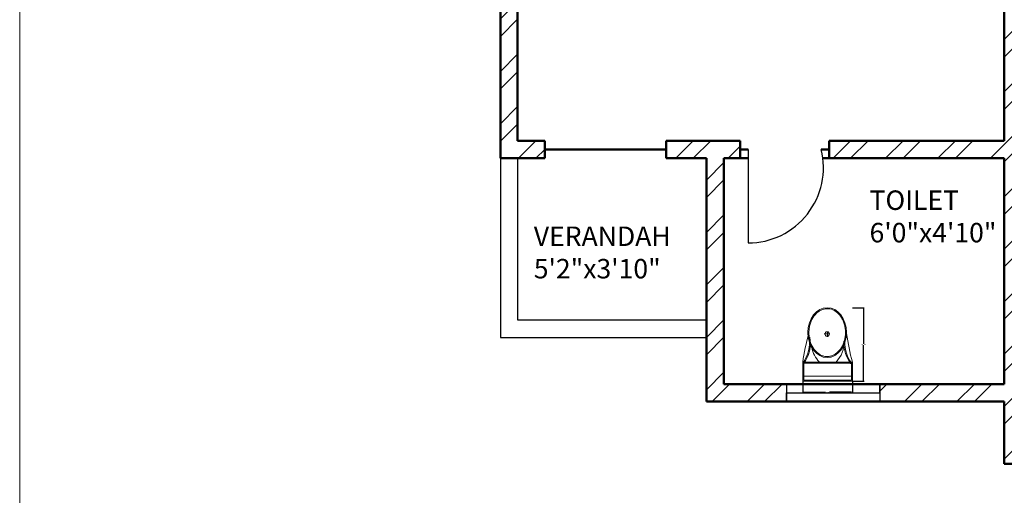
# Model space of a CAD drawing. Units: inches. Extents: x 1901 to 2863, y 888 to 2433.
# Tile 2 of 91: x 1901 to 2154, y 1216 to 1338. Entities that reach past the tile are written whole.
import ezdxf

# ---------------------------------------------------------------- set-up
doc = ezdxf.new("R2010")
doc.units = ezdxf.units.IN
for name, color, linetype, lineweight in [('A-ANNO-DIMS', 2, 'Continuous', 18), ('A-AREA-IDEN', 7, 'Continuous', 18), ('A-DOOR', 4, 'Continuous', 25), ('A-FLOR-FIXT', 9, 'Continuous', 18), ('A-FLOR-HRAL', 41, 'Continuous', 25), ('A-GLAZ', 3, 'Continuous', 25), ('A-WALL', 7, 'Continuous', 50), ('A-WALL-PATT', 8, 'Continuous', 13)]:
    doc.layers.add(name, color=color, linetype=linetype, lineweight=lineweight)
doc.styles.get("Standard").update_dxf_attribs({"font": 'arial.ttf'})
doc.dimstyles.get("Standard").update_dxf_attribs({"dimtxt": 0.18, "dimasz": 0.18, "dimexe": 0.18, "dimexo": 0.0625, "dimgap": 0.09, "dimtad": 0, "dimtih": 1, "dimtoh": 1, "dimdec": 4, "dimzin": 0, "dimdsep": 46, "dimtxsty": 'Standard', "dimcen": 0.09, "dimadec": 0, "dimazin": 0, "dimtfac": 1, "dimtdec": 4, "dimtofl": 0, "dimtmove": 0, "dimatfit": 3, "dimfxl": 1, "dimtolj": 1, "dimtzin": 0, "dimarcsym": 0})

# ---------------------------------------------------------------- blocks, each defined once
blk = doc.blocks.new('A$C31115884')
for p, q in [((258, 466), (258, 523)), ((283, 498), (223, 498)), ((0, 200), (0, 0)), ((520, 200), (0, 200)), ((10, 190), (10, 10)), ((510, 190), (10, 190)), ((510, 10), (510, 190)), ((520, 0), (520, 200)), ((510, 54), (0, 54)), ((10, 10), (510, 10)), ((0, 0), (520, 0))]:
    blk.add_line(p, q)
blk.add_circle((256, 496), 23.6)
for centre, radius, start, end in [((2778, -205), 2807, 165.4549, 171.7133), ((-295, 403), 365, 324.2091, 9.3499), ((-295, 403), 375, 324.2091, 9.3499), ((139, 406), 293, 315.8436, 2.6563), ((806, 403), 365, 170.6501, 215.7909), ((3237, 905), 2807, 188.2867, 194.5451), ((384, 406), 293, 190.2774, 224.1564), ((806, 403), 375, 179.2036, 215.7909)]:
    blk.add_arc(centre, radius, start, end)
blk.add_ellipse((256, 510), major_axis=(0, -261), ratio=0.772727)
blk.add_open_spline([(256, 259), (263, 259), (270, 260), (288, 262), (299, 265), (320, 273), (330, 278), (350, 291), (360, 299), (378, 316), (386, 326), (402, 347), (409, 358), (421, 383), (427, 395), (436, 422), (440, 436), (445, 465), (447, 480), (448, 509), (448, 524), (445, 553), (443, 568), (436, 596), (432, 610), (422, 636), (416, 649), (402, 672), (395, 683), (379, 703), (370, 712), (351, 728), (341, 735), (321, 746), (310, 751), (289, 757), (278, 759), (256, 761), (245, 761), (223, 757), (212, 754), (191, 746), (181, 741), (161, 728), (151, 720), (133, 703), (125, 693), (110, 672), (103, 660), (90, 636), (85, 623), (76, 596), (72, 582), (67, 553), (66, 538), (64, 509), (65, 494), (68, 465), (70, 450), (77, 422), (81, 408), (91, 382), (97, 370), (111, 346), (118, 335), (135, 316), (144, 307), (162, 291), (172, 284), (193, 273), (203, 269), (225, 262), (236, 260), (250, 259), (253, 259), (256, 259)], degree=3, knots=[0, 0, 0, 0, 0.110105, 0.110105, 0.285049, 0.285049, 0.459994, 0.459994, 0.634938, 0.634938, 0.809882, 0.809882, 0.984827, 0.984827, 1.159771, 1.159771, 1.334715, 1.334715, 1.50966, 1.50966, 1.684604, 1.684604, 1.859549, 1.859549, 2.034493, 2.034493, 2.209437, 2.209437, 2.384382, 2.384382, 2.559326, 2.559326, 2.73427, 2.73427, 2.909215, 2.909215, 3.084159, 3.084159, 3.259103, 3.259103, 3.434048, 3.434048, 3.608992, 3.608992, 3.783936, 3.783936, 3.958881, 3.958881, 4.133825, 4.133825, 4.30877, 4.30877, 4.483714, 4.483714, 4.658658, 4.658658, 4.833603, 4.833603, 5.008547, 5.008547, 5.183491, 5.183491, 5.358436, 5.358436, 5.53338, 5.53338, 5.708324, 5.708324, 5.883269, 5.883269, 6.058213, 6.058213, 6.233158, 6.233158, 6.283185, 6.283185, 6.283185, 6.283185])
blk = doc.blocks.new('WIN-24')
for p, q in [((0, 4.5), (0, 0)), ((24, 2.25), (24, 4.5)), ((24, 4.5), (24, 0)), ((0, 0), (0, 2.25)), ((0, 2.25), (24, 2.25))]:
    blk.add_line(p, q)
blk = doc.blocks.new('*D15')
at = {"layer": 'A-ANNO-DIMS', "color": 0, "lineweight": -2, "transparency": 16777216}
for p, q in [((2115.37, 1263.74), (2118.32, 1263.74)), ((2118.14, 1263.56), (2118.14, 1254.48)), ((2118.14, 1245.03), (2118.14, 1254.11)), ((2115.37, 1244.85), (2118.32, 1244.85))]:
    blk.add_line(p, q, dxfattribs=at)
at = {"layer": 'A-ANNO-DIMS', "color": 0, "transparency": 16777216}
for points in [[(2118.11, 1263.56), (2118.17, 1263.56), (2118.14, 1263.74)], [(2118.11, 1245.03), (2118.17, 1245.03), (2118.14, 1244.85)]]:
    blk.add_solid(points, dxfattribs=at)
at = {"layer": 'Defpoints', "color": 0, "transparency": 16777216}
for p in [(2115.3, 1263.74), (2118.14, 1263.74), (2115.3, 1244.85)]:
    blk.add_point(p, dxfattribs=at)
at = {"layer": 'A-ANNO-DIMS', "color": 0, "transparency": 16777216, "insert": (2118.14, 1254.3), "char_height": 0.18, "attachment_point": 5}
blk.add_mtext('\\A1;WC 19 TYP.', dxfattribs=at)
blk = doc.blocks.new('*D16')
at = {"layer": 'A-ANNO-DIMS', "color": 0, "lineweight": -2, "transparency": 16777216}
for p, q in [((2102.56, 1244.79), (2102.56, 1241.84)), ((2115.3, 1244.79), (2115.3, 1241.84)), ((2102.74, 1242.02), (2108.41, 1242.02)), ((2115.12, 1242.02), (2109.45, 1242.02))]:
    blk.add_line(p, q, dxfattribs=at)
at = {"layer": 'A-ANNO-DIMS', "color": 0, "transparency": 16777216}
for points in [[(2102.74, 1242.05), (2102.74, 1241.99), (2102.56, 1242.02)], [(2115.12, 1242.05), (2115.12, 1241.99), (2115.3, 1242.02)]]:
    blk.add_solid(points, dxfattribs=at)
at = {"layer": 'Defpoints', "color": 0, "transparency": 16777216}
for p in [(2102.56, 1244.85), (2115.3, 1244.85), (2115.3, 1242.02)]:
    blk.add_point(p, dxfattribs=at)
at = {"layer": 'A-ANNO-DIMS', "color": 0, "transparency": 16777216, "insert": (2108.93, 1242.02), "char_height": 0.18, "attachment_point": 5}
blk.add_mtext('\\A1;13 TYP.', dxfattribs=at)

msp = doc.modelspace()

# ---------------------------------------------------------------- hatches: boundary and pattern name
at = {"layer": 'A-WALL-PATT'}
h = msp.add_hatch(dxfattribs=at)
h.set_pattern_fill('ANSI32', color=256)
h.paths.add_polyline_path([(2192.5, 2274.13), (2141.26, 2274.13), (2141.26, 2269.63), (2192.5, 2269.63)])
h.paths.add_polyline_path([(2259.93, 2274.13), (2216.5, 2274.13), (2216.5, 2269.63), (2255.43, 2269.63), (2255.43, 2214.63), (2250.81, 2214.63), (2250.81, 2210.13), (2259.93, 2210.13), (2259.93, 2215.13), (2271.76, 2215.13), (2271.76, 2217.38), (2271.76, 2219.63), (2259.93, 2219.63)])
h.paths.add_polyline_path([(2171.43, 2269.63), (2166.93, 2269.63), (2166.93, 2219.63), (2121.24, 2219.63), (2121.24, 2215.13), (2166.93, 2215.13), (2166.93, 2083.13), (2161.81, 2083.13), (2161.81, 2078.63), (2171.43, 2078.63), (2177, 2078.63), (2177, 2080.88), (2177, 2083.13), (2171.43, 2083.13), (2171.43, 2210.13), (2230.91, 2210.13), (2230.91, 2212.38), (2230.91, 2214.63), (2171.43, 2214.63)])
h.paths.add_polyline_path([(2117.26, 2274.13), (2089.43, 2274.13), (2089.43, 2219.63), (2081.14, 2219.63), (2081.14, 2215.13), (2089.43, 2215.13), (2098, 2215.13), (2098, 2217.38), (2098, 2219.63), (2093.93, 2219.63), (2093.93, 2269.63), (2117.26, 2269.63), (2117.26, 2271.88)])
h.paths.add_polyline_path([(2343.43, 2219.63), (2329.29, 2219.63), (2329.29, 2215.13), (2338.93, 2215.13), (2338.93, 2184.74), (2343.43, 2184.74)])
h.paths.add_polyline_path([(2338.93, 2083.13), (2329.29, 2083.13), (2208.97, 2083.13), (2208.97, 2078.63), (2338.93, 2078.63)])
h.paths.add_polyline_path([(2343.43, 2136.74), (2338.93, 2136.74), (2338.93, 1872.63), (2343.43, 1872.63)])
h.paths.add_polyline_path([(2343.43, 1863.63), (2397.68, 1863.63), (2397.68, 1821.63), (2384.14, 1821.63), (2384.14, 1812.63), (2418.33, 1812.63), (2418.33, 1817.13), (2418.33, 1821.63), (2406.68, 1821.63), (2406.68, 1863.63), (2459.5, 1863.63), (2459.5, 1821.63), (2447.14, 1821.63), (2447.14, 1812.63), (2459.5, 1812.63), (2468.5, 1812.63), (2468.5, 1872.63), (2394.43, 1872.63), (2334.43, 1872.63), (2334.43, 1812.63), (2343.43, 1812.63), (2353.25, 1812.63), (2353.25, 1821.63), (2343.43, 1821.63)])
h.paths.add_polyline_path([(2510.01, 1872.63), (2468.5, 1872.63), (2468.5, 1868.13), (2510.01, 1868.13)])
h.paths.add_polyline_path([(2514.01, 1817.13), (2468.5, 1817.13), (2468.5, 1812.63), (2482.11, 1812.63), (2482.11, 1800.61), (2486.61, 1800.61), (2486.61, 1812.63), (2514.01, 1812.63)])
h.paths.add_polyline_path([(2299.25, 1814.88), (2299.25, 1817.13), (2295.93, 1817.13), (2295.93, 1854.17), (2293.68, 1854.17), (2291.43, 1854.17), (2291.43, 1817.13), (2266.11, 1817.13), (2266.11, 1812.63), (2299.25, 1812.63)])
h.paths.add_polyline_path([(2218.11, 1817.13), (2206.46, 1817.13), (2171.43, 1817.13), (2171.43, 1949.13), (2190.1, 1949.13), (2190.1, 1953.63), (2163.47, 1953.63), (2163.47, 1949.13), (2166.93, 1949.13), (2166.93, 1817.13), (2114.3, 1817.13), (2114.3, 1812.63), (2218.11, 1812.63)])
h.paths.add_polyline_path([(2029.43, 1970.92), (2024.93, 1970.92), (2024.93, 1912.72), (2029.43, 1912.72)])
h.paths.add_polyline_path([(2132.3, 1953.63), (2113.93, 1953.63), (2113.93, 1975.89), (2111.68, 1975.89), (2109.43, 1975.89), (2109.43, 1953.63), (2029.43, 1953.63), (2029.43, 1949.13), (2132.3, 1949.13)])
h.paths.add_polyline_path([(2029.43, 1853.61), (2029.31, 1853.61), (2029.31, 1853.61), (2029.43, 1853.61), (2029.43, 1864.72), (2024.93, 1864.72), (2024.93, 1812.63), (2066.3, 1812.63), (2066.3, 1814.88), (2066.3, 1817.13), (2029.43, 1817.13)])
h.paths.add_polyline_path([(2122.93, 2010.09), (2120.68, 2010.09), (2118.43, 2010.09), (2118.43, 2006.13), (2029.43, 2006.13), (2029.43, 2001.63), (2109.43, 2001.63), (2109.43, 1998.04), (2113.93, 1998.04), (2113.93, 2001.63), (2122.93, 2001.63)])
h.paths.add_polyline_path([(2029.43, 2031.38), (2024.93, 2031.38), (2024.93, 1994.92), (2027.18, 1994.92), (2029.43, 1994.92)])
h.paths.add_polyline_path([(2029.43, 2136.74), (2024.93, 2136.74), (2024.93, 2067.38), (2027.18, 2067.38), (2029.43, 2067.38)])
h.paths.add_polyline_path([(2125.62, 2083.13), (2029.43, 2083.13), (2029.43, 2078.63), (2118.43, 2078.63), (2118.43, 2030.71), (2122.93, 2030.71), (2122.93, 2078.63), (2125.62, 2078.63)])
h.paths.add_polyline_path([(2029.43, 2215.13), (2040.47, 2215.13), (2040.47, 2217.38), (2040.47, 2219.63), (2024.93, 2219.63), (2024.93, 2184.74), (2029.43, 2184.74), (2029.43, 2187.78)])
h.paths.add_polyline_path([(2686.43, 2274.13), (2659.28, 2274.13), (2659.28, 2269.63), (2681.93, 2269.63), (2681.93, 2219.63), (2676.82, 2219.63), (2676.82, 2215.13), (2681.93, 2215.13), (2697.01, 2215.13), (2697.01, 2217.38), (2697.01, 2219.63), (2686.43, 2219.63)])
h.paths.add_polyline_path([(2609.93, 2269.63), (2635.28, 2269.63), (2635.28, 2274.13), (2571.43, 2274.13), (2571.43, 2269.63), (2605.43, 2269.63), (2605.43, 2214.63), (2549.1, 2214.63), (2549.1, 2210.13), (2605.43, 2210.13), (2605.43, 2083.13), (2601.01, 2083.13), (2601.01, 2080.88), (2601.01, 2078.63), (2609.93, 2078.63), (2616.16, 2078.63), (2616.16, 2080.88), (2616.16, 2083.13), (2609.93, 2083.13), (2609.93, 2215.13), (2651.46, 2215.13), (2651.46, 2217.38), (2651.46, 2219.63), (2609.93, 2219.63)])
h.paths.add_polyline_path([(2521.43, 2269.63), (2547.43, 2269.63), (2547.43, 2271.88), (2547.43, 2274.13), (2516.93, 2274.13), (2516.93, 2219.63), (2506.41, 2219.63), (2506.41, 2215.13), (2516.93, 2215.13), (2516.93, 2210.13), (2525.4, 2210.13), (2525.4, 2212.38), (2525.4, 2214.63), (2521.43, 2214.63)])
h.paths.add_polyline_path([(2456.01, 2219.63), (2439.43, 2219.63), (2439.43, 2187.89), (2443.93, 2187.89), (2443.93, 2215.13), (2456.01, 2215.13)])
h.paths.add_polyline_path([(2752.93, 2219.63), (2739.48, 2219.63), (2739.48, 2215.13), (2748.43, 2215.13), (2748.43, 2187.89), (2752.93, 2187.89)])
h.paths.add_polyline_path([(2752.93, 2139.89), (2748.43, 2139.89), (2748.43, 2083.13), (2648.42, 2083.13), (2648.42, 2078.63), (2654.93, 2078.63), (2654.93, 2039.44), (2659.43, 2039.44), (2659.43, 2078.63), (2748.43, 2078.63), (2748.43, 2063.43), (2752.93, 2063.43)])
h.paths.add_polyline_path([(2752.93, 2010.63), (2659.43, 2010.63), (2659.43, 2015.65), (2654.93, 2015.65), (2654.93, 2010.63), (2605.43, 2010.63), (2605.43, 1920.97), (2609.93, 1920.97), (2609.93, 2006.13), (2748.43, 2006.13), (2748.43, 1982.47), (2752.93, 1982.47)])
h.paths.add_polyline_path([(2752.93, 2027.43), (2748.43, 2027.43), (2748.43, 2010.63), (2752.93, 2010.63)])
h.paths.add_polyline_path([(2748.43, 1886.13), (2609.93, 1886.13), (2609.93, 1889.72), (2605.43, 1889.72), (2605.43, 1861.26), (2609.93, 1861.26), (2609.93, 1881.63), (2748.43, 1881.63)])
h.paths.add_polyline_path([(2456.86, 2228.83), (2498.4, 2228.83), (2498.4, 2247.49), (2456.86, 2247.49)], flags=9)
h.paths.add_polyline_path([(2038.6, 2237.42), (2080.17, 2237.42), (2080.17, 2256.08), (2038.6, 2256.08)], flags=9)
h.paths.add_polyline_path([(2292.01, 1062.39), (2539.93, 1062.39), (2539.93, 1099.49), (2292.01, 1099.49)], flags=9)
h.paths.add_polyline_path([(2424.91, 1832.25), (2448.51, 1832.25), (2448.51, 1846.68), (2424.91, 1846.68)], flags=25)
h.paths.add_polyline_path([(2359.08, 1832.25), (2382.68, 1832.25), (2382.68, 1846.68), (2359.08, 1846.68)], flags=25)
h.paths.add_polyline_path([(2352.9, 1684.8), (2367.54, 1684.8), (2367.54, 1697.17), (2352.9, 1697.17)], flags=9)
h.paths.add_polyline_path([(2079.29, 1755.83), (2169.02, 1755.83), (2169.02, 1774.37), (2079.29, 1774.37)], flags=9)
h.paths.add_polyline_path([(2404.09, 1373.86), (2404.09, 1463.59), (2385.54, 1463.59), (2385.54, 1373.86)], flags=9)
h.paths.add_polyline_path([(2268.09, 2236.37), (2309.64, 2236.37), (2309.64, 2255.03), (2268.09, 2255.03)], flags=9)
h.paths.add_polyline_path([(2575.96, 1700.95), (2665.7, 1700.95), (2665.7, 1719.5), (2575.96, 1719.5)], flags=9)
h.paths.add_polyline_path([(2302.96, 1878.47), (2329.52, 1878.47), (2329.52, 1888.78), (2302.96, 1888.78)], flags=9)
h.paths.add_polyline_path([(2097.42, 2240.58), (2126.57, 2240.58), (2126.57, 2259.23), (2097.42, 2259.23)], flags=9)
h.paths.add_polyline_path([(2208.72, 2246.12), (2237.88, 2246.12), (2237.88, 2264.78), (2208.72, 2264.78)], flags=9)
h.paths.add_polyline_path([(2038.15, 1925.96), (2076.99, 1925.96), (2076.99, 1944.62), (2038.15, 1944.62)], flags=9)
h.paths.add_polyline_path([(2239.14, 1926.67), (2288.46, 1926.67), (2288.46, 1945.33), (2239.14, 1945.33)], flags=9)
h.paths.add_polyline_path([(2175.43, 2007.33), (2212.36, 2007.33), (2212.36, 2025.99), (2175.43, 2025.99)], flags=9)
h.paths.add_polyline_path([(2225.03, 2091.79), (2263.87, 2091.79), (2263.87, 2110.45), (2225.03, 2110.45)], flags=9)
h.paths.add_polyline_path([(2035.4, 2098.48), (2074.24, 2098.48), (2074.24, 2117.14), (2035.4, 2117.14)], flags=9)
h.paths.add_polyline_path([(2050.1, 2029.21), (2083.26, 2029.21), (2083.26, 2047.87), (2050.1, 2047.87)], flags=9)
h.paths.add_polyline_path([(2069.68, 1956.72), (2098.83, 1956.72), (2098.83, 1975.38), (2069.68, 1975.38)], flags=25)
h.paths.add_polyline_path([(2328.62, 1753.34), (2361.66, 1753.34), (2361.66, 1771.99), (2328.62, 1771.99)], flags=9)
h.paths.add_polyline_path([(2395.16, 2060.89), (2395.16, 2140.65), (2378.68, 2140.65), (2378.68, 2060.89)], flags=9)
h.paths.add_polyline_path([(2463.73, 2059.02), (2492.89, 2059.02), (2492.89, 2077.68), (2463.73, 2077.68)], flags=9)
h.paths.add_polyline_path([(2458.03, 2181.54), (2496.87, 2181.54), (2496.87, 2200.19), (2458.03, 2200.19)], flags=9)
h.paths.add_polyline_path([(2527.58, 2243.07), (2556.73, 2243.07), (2556.73, 2261.73), (2527.58, 2261.73)], flags=9)
h.paths.add_polyline_path([(2694.46, 2232.77), (2736.03, 2232.77), (2736.03, 2251.42), (2694.46, 2251.42)], flags=9)
h.paths.add_polyline_path([(2637.82, 2249.22), (2666.98, 2249.22), (2666.98, 2267.88), (2637.82, 2267.88)], flags=9)
h.paths.add_polyline_path([(2623.69, 2183.54), (2662.53, 2183.54), (2662.53, 2202.2), (2623.69, 2202.2)], flags=9)
h.paths.add_polyline_path([(2691.97, 2021.5), (2725.12, 2021.5), (2725.12, 2040.16), (2691.97, 2040.16)], flags=9)
h.paths.add_polyline_path([(2621.04, 1975.91), (2662.34, 1975.91), (2662.34, 1994.57), (2621.04, 1994.57)], flags=25)
h.paths.add_polyline_path([(2479.03, 1927.62), (2519.84, 1927.62), (2519.84, 1946.28), (2479.03, 1946.28)], flags=9)
h.paths.add_polyline_path([(2670.94, 1849.08), (2716.01, 1849.08), (2716.01, 1867.73), (2670.94, 1867.73)], flags=9)
h.paths.add_polyline_path([(2523.61, 1782.96), (2550.17, 1782.96), (2550.17, 1793.26), (2523.61, 1793.26)], flags=9)
h.paths.add_polyline_path([(2450.84, 1207.33), (2492.39, 1207.33), (2492.39, 1225.99), (2450.84, 1225.99)], flags=9)
h.paths.add_polyline_path([(2527.75, 1203.84), (2556.91, 1203.84), (2556.91, 1222.5), (2527.75, 1222.5)], flags=9)
h.paths.add_polyline_path([(2639.11, 1207.2), (2668.27, 1207.2), (2668.27, 1225.86), (2639.11, 1225.86)], flags=9)
h.paths.add_polyline_path([(2692.59, 1218.97), (2734.17, 1218.97), (2734.17, 1237.62), (2692.59, 1237.62)], flags=9)
h.paths.add_polyline_path([(2669.27, 1366.33), (2708.11, 1366.33), (2708.11, 1384.99), (2669.27, 1384.99)], flags=9)
h.paths.add_polyline_path([(2463.31, 1358.03), (2502.15, 1358.03), (2502.15, 1376.69), (2463.31, 1376.69)], flags=9)
h.paths.add_polyline_path([(2494.72, 1449.96), (2531.65, 1449.96), (2531.65, 1468.62), (2494.72, 1468.62)], flags=9)
h.paths.add_polyline_path([(2675.57, 1422.16), (2708.72, 1422.16), (2708.72, 1440.81), (2675.57, 1440.81)], flags=9)
h.paths.add_polyline_path([(2685.63, 1493.89), (2714.79, 1493.89), (2714.79, 1512.55), (2685.63, 1512.55)], flags=9)
h.paths.add_polyline_path([(2686.8, 1529.91), (2725.65, 1529.91), (2725.65, 1548.57), (2686.8, 1548.57)], flags=9)
h.paths.add_polyline_path([(2503.65, 1537.99), (2552.97, 1537.99), (2552.97, 1556.65), (2503.65, 1556.65)], flags=9)
h.paths.add_polyline_path([(2291.71, 1643.5), (2318.28, 1643.5), (2318.28, 1653.81), (2291.71, 1653.81)], flags=9)
h.paths.add_polyline_path([(2450.63, 1610.52), (2477.19, 1610.52), (2477.19, 1620.82), (2450.63, 1620.82)], flags=9)
h.paths.add_polyline_path([(2359.99, 1551.81), (2422.25, 1551.81), (2422.25, 1562.12), (2359.99, 1562.12)], flags=9)
h.paths.add_polyline_path([(2280.11, 1249.01), (2321.65, 1249.01), (2321.65, 1267.66), (2280.11, 1267.66)], flags=9)
h.paths.add_polyline_path([(2164.06, 1274.23), (2193.22, 1274.23), (2193.22, 1292.89), (2164.06, 1292.89)], flags=9)
h.paths.add_polyline_path([(2118.21, 1277.69), (2151.25, 1277.69), (2151.25, 1296.35), (2118.21, 1296.35)], flags=9)
h.paths.add_polyline_path([(2031.95, 1268.53), (2073.52, 1268.53), (2073.52, 1287.19), (2031.95, 1287.19)], flags=9)
h.paths.add_polyline_path([(2050.2, 1409.08), (2089.04, 1409.08), (2089.04, 1427.74), (2050.2, 1427.74)], flags=9)
h.paths.add_polyline_path([(2243.74, 1421.03), (2282.58, 1421.03), (2282.58, 1439.69), (2243.74, 1439.69)], flags=9)
h.paths.add_polyline_path([(2190.75, 1509.77), (2231.56, 1509.77), (2231.56, 1528.43), (2190.75, 1528.43)], flags=9)
h.paths.add_polyline_path([(2058.39, 1475.42), (2091.55, 1475.42), (2091.55, 1494.07), (2058.39, 1494.07)], flags=9)
h.paths.add_polyline_path([(2062.45, 1553.09), (2091.6, 1553.09), (2091.6, 1571.75), (2062.45, 1571.75)], flags=9)
h.paths.add_polyline_path([(2219.52, 1590.37), (2266.15, 1590.37), (2266.15, 1609.02), (2219.52, 1609.02)], flags=9)
h.paths.add_polyline_path([(2041.07, 1584.19), (2079.91, 1584.19), (2079.91, 1602.85), (2041.07, 1602.85)], flags=9)
h = msp.add_hatch(dxfattribs=at)
h.set_pattern_fill('ANSI32', color=256)
h.paths.add_polyline_path([(2443.93, 2139.89), (2439.43, 2139.89), (2439.43, 2069.35), (2441.68, 2069.35), (2443.93, 2069.35), (2443.93, 2078.63), (2521.93, 2078.63), (2521.93, 2075.07), (2524.18, 2075.07), (2526.43, 2075.07), (2526.43, 2078.63), (2571.75, 2078.63), (2571.75, 2080.88), (2571.75, 2083.13), (2443.93, 2083.13)])
h.paths.add_polyline_path([(2526.43, 2054.63), (2524.18, 2054.63), (2521.93, 2054.63), (2521.93, 2030.63), (2443.93, 2030.63), (2443.93, 2045.35), (2439.43, 2045.35), (2439.43, 1983.87), (2443.93, 1983.87), (2443.93, 2026.13), (2521.93, 2026.13), (2526.43, 2026.13)])
h.paths.add_polyline_path([(2443.93, 1923.87), (2439.43, 1923.87), (2439.43, 1872.63), (2443.93, 1872.63)])
h.paths.add_polyline_path([(2636.23, 1766.13), (2609.93, 1766.13), (2609.93, 1779.79), (2605.43, 1779.79), (2605.43, 1766.13), (2486.61, 1766.13), (2486.61, 1770.67), (2482.11, 1770.67), (2482.11, 1766.13), (2482.11, 1761.63), (2636.23, 1761.63), (2636.23, 1763.88)])
h.paths.add_polyline_path([(2519.54, 1663.38), (2519.54, 1665.63), (2494.93, 1665.63), (2481.83, 1665.63), (2481.83, 1663.38), (2481.83, 1661.13), (2490.43, 1661.13), (2490.43, 1640.16), (2494.93, 1640.16), (2494.93, 1661.13), (2519.54, 1661.13)])
h.paths.add_polyline_path([(2443.93, 1712.13), (2443.93, 1716.63), (2414.46, 1716.63), (2414.46, 1712.13), (2439.43, 1712.13), (2439.43, 1545.51), (2443.93, 1545.51), (2443.93, 1661.13), (2448.47, 1661.13), (2448.47, 1665.63), (2443.93, 1665.63)])
h.paths.add_polyline_path([(2343.43, 1712.13), (2365.52, 1712.13), (2365.52, 1714.38), (2365.52, 1716.63), (2333.87, 1716.63), (2333.87, 1714.38), (2333.87, 1712.13), (2338.93, 1712.13), (2338.93, 1575.63), (2338.93, 1545.51), (2343.43, 1545.51), (2343.43, 1547.51), (2343.43, 1580.13)])
h.paths.add_polyline_path([(2752.93, 1665.63), (2579.54, 1665.63), (2579.54, 1661.13), (2615.93, 1661.13), (2615.93, 1529.13), (2598.93, 1529.13), (2598.93, 1524.63), (2623.13, 1524.63), (2623.13, 1526.88), (2623.13, 1529.13), (2620.43, 1529.13), (2620.43, 1661.13), (2748.43, 1661.13), (2748.43, 1633.5), (2752.93, 1633.5)])
h.paths.add_polyline_path([(2752.93, 1419.93), (2748.43, 1419.93), (2748.43, 1400.13), (2659.43, 1400.13), (2659.43, 1444.33), (2657.18, 1444.33), (2654.93, 1444.33), (2654.93, 1400.13), (2643.65, 1400.13), (2643.65, 1395.63), (2748.43, 1395.63), (2748.43, 1364.04), (2752.93, 1364.04)])
h.paths.add_polyline_path([(2752.93, 1492.88), (2748.43, 1492.88), (2748.43, 1476.63), (2667.43, 1476.63), (2667.43, 1479.71), (2665.18, 1479.71), (2662.93, 1479.71), (2662.93, 1476.63), (2654.93, 1476.63), (2654.93, 1469.54), (2659.43, 1469.54), (2659.43, 1472.13), (2748.43, 1472.13), (2748.43, 1455.93), (2752.93, 1455.93)])
h.paths.add_polyline_path([(2752.93, 1304.04), (2748.43, 1304.04), (2748.43, 1263.63), (2738.66, 1263.63), (2738.66, 1259.13), (2752.93, 1259.13)])
h.paths.add_polyline_path([(2685.93, 1259.13), (2695.49, 1259.13), (2695.49, 1261.38), (2695.49, 1263.63), (2677.84, 1263.63), (2677.84, 1261.38), (2677.84, 1259.13), (2681.43, 1259.13), (2681.43, 1203.63), (2653.28, 1203.63), (2653.28, 1199.13), (2685.93, 1199.13), (2685.93, 1203.63)])
h.paths.add_polyline_path([(2609.43, 1395.63), (2611.85, 1395.63), (2611.85, 1400.13), (2598.89, 1400.13), (2598.89, 1397.88), (2598.89, 1395.63), (2604.93, 1395.63), (2604.93, 1268.13), (2554.73, 1268.13), (2554.73, 1265.88), (2554.73, 1263.63), (2604.93, 1263.63), (2604.93, 1203.63), (2571.31, 1203.63), (2571.31, 1199.13), (2604.93, 1199.13), (2629.28, 1199.13), (2629.28, 1201.38), (2629.28, 1203.63), (2609.43, 1203.63), (2609.43, 1258.63), (2609.43, 1259.13), (2654.8, 1259.13), (2654.8, 1263.63), (2609.43, 1263.63)])
h.paths.add_polyline_path([(2443.93, 1304.04), (2439.43, 1304.04), (2439.43, 1259.13), (2443.93, 1259.13), (2456.16, 1259.13), (2456.16, 1261.38), (2456.16, 1263.63), (2443.93, 1263.63)])
h.paths.add_polyline_path([(2525.43, 1263.63), (2531.78, 1263.63), (2531.78, 1268.13), (2520.93, 1268.13), (2520.93, 1263.63), (2511.41, 1263.63), (2511.41, 1259.13), (2520.93, 1259.13), (2520.93, 1199.13), (2547.31, 1199.13), (2547.31, 1201.38), (2547.31, 1203.63), (2525.43, 1203.63)])
h.paths.add_polyline_path([(2443.93, 1434.84), (2439.43, 1434.84), (2439.43, 1364.04), (2441.68, 1364.04), (2443.93, 1364.04)])
h.paths.add_polyline_path([(2567.13, 1400.13), (2443.93, 1400.13), (2443.93, 1395.63), (2567.13, 1395.63)])
h.paths.add_polyline_path([(2443.93, 1545.51), (2439.43, 1545.51), (2439.43, 1494.84), (2443.93, 1494.84)])
h.paths.add_polyline_path([(2494.93, 1553.35), (2492.68, 1553.35), (2490.43, 1553.35), (2490.43, 1524.63), (2494.93, 1524.63), (2525.94, 1524.63), (2525.94, 1526.88), (2525.94, 1529.13), (2494.93, 1529.13)])
h.paths.add_polyline_path([(2752.93, 1573.5), (2748.43, 1573.5), (2748.43, 1529.13), (2657.76, 1529.13), (2657.76, 1524.63), (2662.93, 1524.63), (2662.93, 1498.63), (2667.43, 1498.63), (2667.43, 1524.63), (2748.43, 1524.63), (2748.43, 1516.88), (2752.93, 1516.88)])
h.paths.add_polyline_path([(2038.6, 2237.42), (2080.17, 2237.42), (2080.17, 2256.08), (2038.6, 2256.08)], flags=9)
h.paths.add_polyline_path([(2292.01, 1062.39), (2539.93, 1062.39), (2539.93, 1099.49), (2292.01, 1099.49)], flags=9)
h.paths.add_polyline_path([(2424.91, 1832.25), (2448.51, 1832.25), (2448.51, 1846.68), (2424.91, 1846.68)], flags=9)
h.paths.add_polyline_path([(2359.08, 1832.25), (2382.68, 1832.25), (2382.68, 1846.68), (2359.08, 1846.68)], flags=9)
h.paths.add_polyline_path([(2352.9, 1684.8), (2367.54, 1684.8), (2367.54, 1697.17), (2352.9, 1697.17)], flags=9)
h.paths.add_polyline_path([(2079.29, 1755.83), (2169.02, 1755.83), (2169.02, 1774.37), (2079.29, 1774.37)], flags=9)
h.paths.add_polyline_path([(2404.09, 1373.86), (2404.09, 1463.59), (2385.54, 1463.59), (2385.54, 1373.86)], flags=9)
h.paths.add_polyline_path([(2268.09, 2236.37), (2309.64, 2236.37), (2309.64, 2255.03), (2268.09, 2255.03)], flags=9)
h.paths.add_polyline_path([(2575.96, 1700.95), (2665.7, 1700.95), (2665.7, 1719.5), (2575.96, 1719.5)], flags=9)
h.paths.add_polyline_path([(2302.96, 1878.47), (2329.52, 1878.47), (2329.52, 1888.78), (2302.96, 1888.78)], flags=9)
h.paths.add_polyline_path([(2097.42, 2240.58), (2126.57, 2240.58), (2126.57, 2259.23), (2097.42, 2259.23)], flags=9)
h.paths.add_polyline_path([(2208.72, 2246.12), (2237.88, 2246.12), (2237.88, 2264.78), (2208.72, 2264.78)], flags=9)
h.paths.add_polyline_path([(2038.15, 1925.96), (2076.99, 1925.96), (2076.99, 1944.62), (2038.15, 1944.62)], flags=9)
h.paths.add_polyline_path([(2239.14, 1926.67), (2288.46, 1926.67), (2288.46, 1945.33), (2239.14, 1945.33)], flags=9)
h.paths.add_polyline_path([(2175.43, 2007.33), (2212.36, 2007.33), (2212.36, 2025.99), (2175.43, 2025.99)], flags=9)
h.paths.add_polyline_path([(2225.03, 2091.79), (2263.87, 2091.79), (2263.87, 2110.45), (2225.03, 2110.45)], flags=9)
h.paths.add_polyline_path([(2035.4, 2098.48), (2074.24, 2098.48), (2074.24, 2117.14), (2035.4, 2117.14)], flags=9)
h.paths.add_polyline_path([(2050.1, 2029.21), (2083.26, 2029.21), (2083.26, 2047.87), (2050.1, 2047.87)], flags=9)
h.paths.add_polyline_path([(2069.68, 1956.72), (2098.83, 1956.72), (2098.83, 1975.38), (2069.68, 1975.38)], flags=9)
h.paths.add_polyline_path([(2328.62, 1753.34), (2361.66, 1753.34), (2361.66, 1771.99), (2328.62, 1771.99)], flags=9)
h.paths.add_polyline_path([(2395.16, 2060.89), (2395.16, 2140.65), (2378.68, 2140.65), (2378.68, 2060.89)], flags=9)
h.paths.add_polyline_path([(2463.73, 2059.02), (2492.89, 2059.02), (2492.89, 2077.68), (2463.73, 2077.68)], flags=9)
h.paths.add_polyline_path([(2458.03, 2181.54), (2496.87, 2181.54), (2496.87, 2200.19), (2458.03, 2200.19)], flags=9)
h.paths.add_polyline_path([(2456.86, 2228.83), (2498.4, 2228.83), (2498.4, 2247.49), (2456.86, 2247.49)], flags=9)
h.paths.add_polyline_path([(2527.58, 2243.07), (2556.73, 2243.07), (2556.73, 2261.73), (2527.58, 2261.73)], flags=9)
h.paths.add_polyline_path([(2694.46, 2232.77), (2736.03, 2232.77), (2736.03, 2251.42), (2694.46, 2251.42)], flags=9)
h.paths.add_polyline_path([(2637.82, 2249.22), (2666.98, 2249.22), (2666.98, 2267.88), (2637.82, 2267.88)], flags=9)
h.paths.add_polyline_path([(2623.69, 2183.54), (2662.53, 2183.54), (2662.53, 2202.2), (2623.69, 2202.2)], flags=9)
h.paths.add_polyline_path([(2691.97, 2021.5), (2725.12, 2021.5), (2725.12, 2040.16), (2691.97, 2040.16)], flags=9)
h.paths.add_polyline_path([(2621.04, 1975.91), (2662.34, 1975.91), (2662.34, 1994.57), (2621.04, 1994.57)], flags=9)
h.paths.add_polyline_path([(2479.03, 1927.62), (2519.84, 1927.62), (2519.84, 1946.28), (2479.03, 1946.28)], flags=9)
h.paths.add_polyline_path([(2670.94, 1849.08), (2716.01, 1849.08), (2716.01, 1867.73), (2670.94, 1867.73)], flags=9)
h.paths.add_polyline_path([(2523.61, 1782.96), (2550.17, 1782.96), (2550.17, 1793.26), (2523.61, 1793.26)], flags=9)
h.paths.add_polyline_path([(2450.84, 1207.33), (2492.39, 1207.33), (2492.39, 1225.99), (2450.84, 1225.99)], flags=9)
h.paths.add_polyline_path([(2527.75, 1203.84), (2556.91, 1203.84), (2556.91, 1222.5), (2527.75, 1222.5)], flags=9)
h.paths.add_polyline_path([(2639.11, 1207.2), (2668.27, 1207.2), (2668.27, 1225.86), (2639.11, 1225.86)], flags=9)
h.paths.add_polyline_path([(2692.59, 1218.97), (2734.17, 1218.97), (2734.17, 1237.62), (2692.59, 1237.62)], flags=9)
h.paths.add_polyline_path([(2669.27, 1366.33), (2708.11, 1366.33), (2708.11, 1384.99), (2669.27, 1384.99)], flags=25)
h.paths.add_polyline_path([(2463.31, 1358.03), (2502.15, 1358.03), (2502.15, 1376.69), (2463.31, 1376.69)], flags=9)
h.paths.add_polyline_path([(2494.72, 1449.96), (2531.65, 1449.96), (2531.65, 1468.62), (2494.72, 1468.62)], flags=9)
h.paths.add_polyline_path([(2675.57, 1422.16), (2708.72, 1422.16), (2708.72, 1440.81), (2675.57, 1440.81)], flags=25)
h.paths.add_polyline_path([(2685.63, 1493.89), (2714.79, 1493.89), (2714.79, 1512.55), (2685.63, 1512.55)], flags=9)
h.paths.add_polyline_path([(2686.8, 1529.91), (2725.65, 1529.91), (2725.65, 1548.57), (2686.8, 1548.57)], flags=25)
h.paths.add_polyline_path([(2503.65, 1537.99), (2552.97, 1537.99), (2552.97, 1556.65), (2503.65, 1556.65)], flags=9)
h.paths.add_polyline_path([(2291.71, 1643.5), (2318.28, 1643.5), (2318.28, 1653.81), (2291.71, 1653.81)], flags=9)
h.paths.add_polyline_path([(2450.63, 1610.52), (2477.19, 1610.52), (2477.19, 1620.82), (2450.63, 1620.82)], flags=9)
h.paths.add_polyline_path([(2359.99, 1551.81), (2422.25, 1551.81), (2422.25, 1562.12), (2359.99, 1562.12)], flags=9)
h.paths.add_polyline_path([(2280.11, 1249.01), (2321.65, 1249.01), (2321.65, 1267.66), (2280.11, 1267.66)], flags=9)
h.paths.add_polyline_path([(2164.06, 1274.23), (2193.22, 1274.23), (2193.22, 1292.89), (2164.06, 1292.89)], flags=9)
h.paths.add_polyline_path([(2118.21, 1277.69), (2151.25, 1277.69), (2151.25, 1296.35), (2118.21, 1296.35)], flags=9)
h.paths.add_polyline_path([(2031.95, 1268.53), (2073.52, 1268.53), (2073.52, 1287.19), (2031.95, 1287.19)], flags=9)
h.paths.add_polyline_path([(2050.2, 1409.08), (2089.04, 1409.08), (2089.04, 1427.74), (2050.2, 1427.74)], flags=9)
h.paths.add_polyline_path([(2243.74, 1421.03), (2282.58, 1421.03), (2282.58, 1439.69), (2243.74, 1439.69)], flags=9)
h.paths.add_polyline_path([(2190.75, 1509.77), (2231.56, 1509.77), (2231.56, 1528.43), (2190.75, 1528.43)], flags=9)
h.paths.add_polyline_path([(2058.39, 1475.42), (2091.55, 1475.42), (2091.55, 1494.07), (2058.39, 1494.07)], flags=9)
h.paths.add_polyline_path([(2062.45, 1553.09), (2091.6, 1553.09), (2091.6, 1571.75), (2062.45, 1571.75)], flags=9)
h.paths.add_polyline_path([(2219.52, 1590.37), (2266.15, 1590.37), (2266.15, 1609.02), (2219.52, 1609.02)], flags=9)
h.paths.add_polyline_path([(2041.07, 1584.19), (2079.91, 1584.19), (2079.91, 1602.85), (2041.07, 1602.85)], flags=9)
h = msp.add_hatch(dxfattribs=at)
h.set_pattern_fill('ANSI32', color=256)
h.paths.add_polyline_path([(2182.93, 1716.63), (2024.93, 1716.63), (2024.93, 1681.7), (2029.33, 1681.7), (2029.33, 1712.13), (2154.33, 1712.13), (2154.33, 1580.13), (2148.52, 1580.13), (2148.52, 1577.88), (2148.52, 1575.63), (2194.93, 1575.63), (2194.93, 1580.13), (2158.83, 1580.13), (2158.83, 1712.13), (2182.93, 1712.13)])
h.paths.add_polyline_path([(2301.07, 1716.63), (2242.93, 1716.63), (2242.93, 1712.13), (2283.83, 1712.13), (2283.83, 1685.54), (2288.33, 1685.54), (2288.33, 1712.13), (2301.07, 1712.13)])
h.paths.add_polyline_path([(2288.33, 1600.41), (2286.08, 1600.41), (2283.83, 1600.41), (2283.83, 1580.13), (2270.6, 1580.13), (2270.6, 1575.63), (2288.33, 1575.63)])
h.paths.add_polyline_path([(2295.93, 1953.63), (2271.45, 1953.63), (2271.45, 1949.13), (2291.43, 1949.13), (2291.43, 1941.24), (2295.93, 1941.24)])
h.paths.add_polyline_path([(2098.38, 1244.13), (2082.33, 1244.13), (2082.33, 1302.13), (2086.52, 1302.13), (2086.52, 1306.63), (2067.46, 1306.63), (2067.46, 1302.13), (2077.83, 1302.13), (2077.83, 1239.63), (2098.38, 1239.63), (2098.38, 1241.88)])
h.paths.add_polyline_path([(2217.31, 1306.63), (2158.83, 1306.63), (2158.83, 1451.63), (2162.72, 1451.63), (2162.72, 1453.88), (2162.72, 1456.13), (2154.33, 1456.13), (2154.33, 1443.13), (2151.91, 1443.13), (2151.91, 1438.63), (2154.33, 1438.63), (2154.33, 1306.63), (2109.31, 1306.63), (2109.31, 1304.38), (2109.31, 1302.13), (2154.33, 1302.13), (2154.33, 1244.13), (2122.38, 1244.13), (2122.38, 1239.63), (2154.33, 1239.63), (2154.33, 1223.63), (2163.33, 1223.63), (2181.01, 1223.63), (2181.01, 1225.88), (2181.01, 1228.13), (2163.33, 1228.13), (2163.33, 1258.22), (2158.83, 1258.22), (2158.83, 1302.13), (2217.31, 1302.13)])
h.paths.add_polyline_path([(2259.99, 1306.63), (2238.3, 1306.63), (2238.3, 1304.38), (2238.3, 1302.13), (2242.83, 1302.13), (2242.83, 1228.13), (2205.01, 1228.13), (2205.01, 1223.63), (2247.33, 1223.63), (2247.33, 1302.13), (2259.99, 1302.13), (2259.99, 1304.38)])
h.paths.add_polyline_path([(2343.43, 1361.7), (2338.93, 1361.7), (2338.93, 1306.63), (2322.38, 1306.63), (2322.38, 1302.13), (2343.43, 1302.13)])
h.paths.add_polyline_path([(2343.43, 1470.4), (2338.93, 1470.4), (2338.93, 1456.13), (2193.73, 1456.13), (2193.73, 1453.88), (2193.73, 1451.63), (2338.93, 1451.63), (2338.93, 1421.7), (2343.43, 1421.7)])
h.paths.add_polyline_path([(2343.43, 1545.51), (2338.93, 1545.51), (2338.93, 1530.4), (2343.43, 1530.4)])
h.paths.add_polyline_path([(2029.33, 1466.83), (2024.93, 1466.83), (2024.93, 1409.82), (2029.33, 1409.82)])
h.paths.add_polyline_path([(2122.84, 1440.88), (2122.84, 1443.13), (2121.83, 1443.13), (2121.83, 1498.18), (2119.58, 1498.18), (2117.33, 1498.18), (2117.33, 1443.13), (2029.33, 1443.13), (2029.33, 1438.63), (2122.84, 1438.63)])
h.paths.add_polyline_path([(2029.33, 1543.05), (2024.93, 1543.05), (2024.93, 1502.83), (2029.33, 1502.83)])
h.paths.add_polyline_path([(2029.33, 1621.7), (2024.93, 1621.7), (2024.93, 1567.05), (2027.13, 1567.05), (2029.33, 1567.05), (2029.33, 1575.63), (2109.33, 1575.63), (2109.33, 1554.71), (2113.83, 1554.71), (2113.83, 1575.63), (2115.8, 1575.63), (2115.8, 1577.88), (2115.8, 1580.13), (2029.33, 1580.13)])
h.paths.add_polyline_path([(2121.83, 1527.63), (2117.33, 1527.63), (2113.83, 1527.63), (2113.83, 1533.01), (2111.58, 1533.01), (2109.33, 1533.01), (2109.33, 1527.63), (2029.33, 1527.63), (2029.33, 1523.13), (2117.33, 1523.13), (2117.33, 1519.43), (2121.83, 1519.43)])
h.paths.add_polyline_path([(2029.33, 1349.82), (2024.93, 1349.82), (2024.93, 1302.13), (2036.28, 1302.13), (2036.28, 1306.63), (2029.33, 1306.63)])

# ---------------------------------------------------------------- linework, layer by layer
at = {"layer": 'A-DOOR'}
msp.add_line((2088.52, 1304.38), (2088.52, 1280.38), dxfattribs=at)
msp.add_arc((2088.52, 1299.73), 19.35, 270, 13.9031, dxfattribs=at)
at = {"layer": 'A-FLOR-FIXT'}
msp.add_lwpolyline([(1901.45, 2433.12), (2863.43, 2433.12), (2863.43, 961.82), (1901.45, 961.82)], close=True, dxfattribs=at)
at = {"layer": 'A-FLOR-HRAL'}
for p, q in [((2024.93, 1302.13), (2024.93, 1256.13)), ((2029.33, 1302.13), (2029.33, 1260.63)), ((2029.33, 1260.63), (2077.83, 1260.63)), ((2024.93, 1256.13), (2077.83, 1256.13))]:
    msp.add_line(p, q, dxfattribs=at)
at = {"layer": 'A-WALL'}
for p, q in [((2024.93, 1716.63), (2024.93, 1302.13)), ((2029.33, 1575.63), (2029.33, 1306.63)), ((2154.33, 1438.63), (2154.33, 1306.63)), ((2036.28, 1306.63), (2029.33, 1306.63)), ((2036.28, 1302.13), (2036.28, 1306.63)), ((2036.28, 1306.63), (2036.28, 1304.38)), ((2067.46, 1304.38), (2067.46, 1306.63)), ((2067.46, 1306.63), (2067.46, 1302.13)), ((2086.52, 1306.63), (2067.46, 1306.63)), ((2086.52, 1302.13), (2086.52, 1306.63)), ((2086.52, 1306.63), (2086.52, 1304.38)), ((2154.33, 1306.63), (2109.31, 1306.63)), ((2109.31, 1302.13), (2109.31, 1306.63)), ((2109.31, 1306.63), (2109.31, 1304.38)), ((2036.28, 1304.38), (2067.46, 1304.38)), ((2086.52, 1304.38), (2088.52, 1304.38)), ((2109.31, 1304.38), (2107.31, 1304.38)), ((2036.28, 1302.13), (2024.93, 1302.13)), ((2077.83, 1302.13), (2067.46, 1302.13)), ((2077.83, 1302.13), (2077.83, 1239.63)), ((2082.33, 1302.13), (2082.33, 1244.13)), ((2088.52, 1302.13), (2082.33, 1302.13)), ((2154.33, 1302.13), (2107.72, 1302.13)), ((2154.33, 1302.13), (2154.33, 1244.13)), ((2154.33, 1302.13), (2154.33, 1244.13)), ((2077.83, 1244.13), (2077.83, 1239.63)), ((2154.33, 1244.13), (2082.33, 1244.13)), ((2077.83, 1239.63), (2154.33, 1239.63)), ((2154.33, 1239.63), (2154.33, 1223.63)), ((2247.33, 1223.63), (2154.33, 1223.63)), ((2154.33, 1223.63), (2163.33, 1223.63))]:
    msp.add_line(p, q, dxfattribs=at)

# ---------------------------------------------------------------- block references
at = {"layer": 'A-FLOR-FIXT', "xscale": 0.0245149588751191, "yscale": 0.0245149588751191, "zscale": 0.0245149588751191}
msp.add_blockref('A$C31115884', (2102.56, 1244.85), dxfattribs=at)
at = {"layer": 'A-GLAZ'}
msp.add_blockref('WIN-24', (2098.38, 1239.63), dxfattribs=at)

# ---------------------------------------------------------------- texts
at = {"layer": 'A-AREA-IDEN', "char_height": 5, "attachment_point": 1}
for s, width, insert in [('TOILET\\P6\'0"x4\'10"', 86.5262, (2119.72, 1293.87)), ('VERANDAH\\P5\'2"x3\'10"', 76.4633, (2033.49, 1284.61))]:
    msp.add_mtext_dynamic_manual_height_columns(s, width=width, gutter_width=12.5, heights=[0], dxfattribs=dict(at, insert=insert))

# ---------------------------------------------------------------- dimensions: what is measured, and where the dimension line sits
at = {"layer": 'A-ANNO-DIMS'}
dim = msp.add_linear_dim(base=(2118.14, 1263.74), p1=(2115.3, 1244.85), p2=(2115.3, 1263.74), angle=90, text='WC <> TYP.', dimstyle='Standard', override={"dimdec": 0, "dimlfac": 1, "dimrnd": 0, "dimzin": 0, "dimdsep": 46, "dimlunit": 2}, dxfattribs=at)
dim.commit()
dim.dimension.update_dxf_attribs({"geometry": '*D15', "text_midpoint": (2118.14, 1254.3)})
dim = msp.add_linear_dim(base=(2115.3, 1242.02), p1=(2102.56, 1244.85), p2=(2115.3, 1244.85), text='<> TYP.', dimstyle='Standard', override={"dimdec": 0, "dimlfac": 1, "dimrnd": 0, "dimzin": 0, "dimdsep": 46, "dimlunit": 2}, dxfattribs=at)
dim.commit()
dim.dimension.update_dxf_attribs({"geometry": '*D16', "text_midpoint": (2108.93, 1242.02)})

doc.saveas('drawing.dxf')
